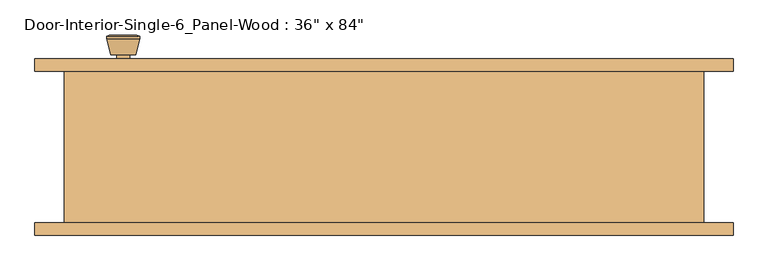
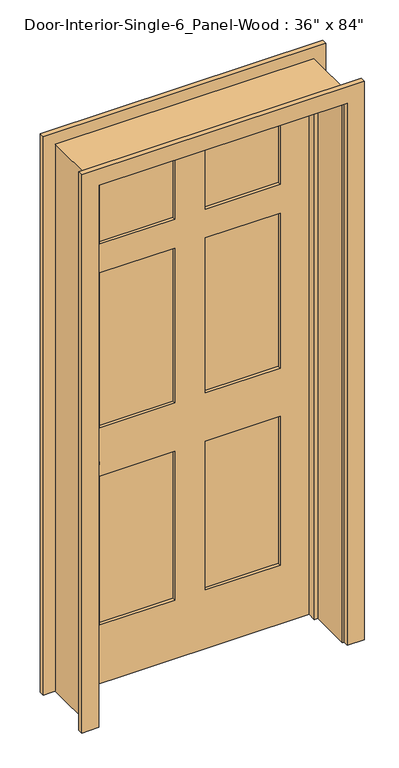
"""IFC4 building model written with IfcOpenShell, lengths in millimetres: door geometry."""

from ifc_helpers import new_model, si_unit, point, frame, frame_2d, origin, place, context, project, spatial, polyline, circle_curve, trimmed, segment, composite_curve, outline, extrude, faceted_brep, source, transform, mapped, element, save
from ifc_brep_helpers import plane_surface, cylinder_surface, revolved_surface, advanced_brep


def door_d86b6c54(model_context):
    return source(origin(), model_context, "Body", "SolidModel", [
        advanced_brep(
        [(-393.7, 70.2, 914.4), (-383.7, 70.2, 914.4), (-403.7, 70.2, 914.4), (-373.2241324, 21.2, 914.4), (-393.7, 21.2, 914.4), (-414.1758676, 21.2, 914.4), (-368.7, 23.0278681, 914.4), (-418.7, 23.0278681, 914.4), (-368.7, 26.4915463, 914.4), (-418.7, 26.4915463, 914.4), (-375.063764, 51.2, 914.4), (-412.336236, 51.2, 914.4), (-383.7, 51.2, 914.4), (-403.7, 51.2, 914.4)],
        [
            (0, 1),
            (1, 2, circle_curve(frame((-393.7, 70.2, 914.4), z_axis=(0.0, 1.0, 0.0), x_axis=(-1.0, 0.0, 0.0)), 10.0)),
            (2, 0),
            (2, 1, circle_curve(frame((-393.7, 70.2, 914.4), z_axis=(0.0, 1.0, 0.0), x_axis=(-1.0, 0.0, 0.0)), 10.0)),
            (3, 4),
            (4, 5),
            (5, 3, circle_curve(frame((-393.7, 21.2, 914.4), z_axis=(0.0, -1.0, 0.0), x_axis=(-1.0, 0.0, 0.0)), 20.4758676)),
            (3, 5, circle_curve(frame((-393.7, 21.2, 914.4), z_axis=(0.0, -1.0, 0.0), x_axis=(-1.0, 0.0, 0.0)), 20.4758676)),
            (6, 3),
            (5, 7),
            (7, 6, circle_curve(frame((-393.7, 23.0278681, 914.4), z_axis=(0.0, -1.0, 0.0), x_axis=(-1.0, 0.0, 0.0)), 25.0)),
            (6, 7, circle_curve(frame((-393.7, 23.0278681, 914.4), z_axis=(0.0, -1.0, 0.0), x_axis=(-1.0, 0.0, 0.0)), 25.0)),
            (8, 6),
            (7, 9),
            (9, 8, circle_curve(frame((-393.7, 26.4915463, 914.4), z_axis=(0.0, -1.0, 0.0), x_axis=(-1.0, 0.0, 0.0)), 25.0)),
            (8, 9, circle_curve(frame((-393.7, 26.4915463, 914.4), z_axis=(0.0, -1.0, 0.0), x_axis=(-1.0, 0.0, 0.0)), 25.0)),
            (10, 8),
            (9, 11),
            (11, 10, circle_curve(frame((-393.7, 51.2, 914.4), z_axis=(0.0, -1.0, 0.0), x_axis=(-1.0, 0.0, 0.0)), 18.636236)),
            (10, 11, circle_curve(frame((-393.7, 51.2, 914.4), z_axis=(0.0, -1.0, 0.0), x_axis=(-1.0, 0.0, 0.0)), 18.636236)),
            (12, 10),
            (11, 13),
            (13, 12, circle_curve(frame((-393.7, 51.2, 914.4), z_axis=(0.0, -1.0, 0.0), x_axis=(-1.0, 0.0, 0.0)), 10.0)),
            (12, 13, circle_curve(frame((-393.7, 51.2, 914.4), z_axis=(0.0, -1.0, 0.0), x_axis=(-1.0, 0.0, 0.0)), 10.0)),
            (1, 12),
            (13, 2),
        ],
        [
            plane_surface(frame((-393.7, 70.2, 914.4), z_axis=(0.0, 1.0, 0.0), x_axis=(-1.0, 0.0, 0.0))),
            plane_surface(frame((-393.7, 21.2, 914.4), z_axis=(0.0, -1.0, 0.0), x_axis=(-1.0, 0.0, 0.0))),
            revolved_surface(polyline([(-414.1758676, 21.2, 914.4), (-418.7, 23.0278681, 914.4)]), (-393.7, 70.2, 914.4), (0.0, 1.0, 0.0)),
            cylinder_surface(frame((-393.7, 70.2, 914.4), z_axis=(0.0, 1.0, 0.0), x_axis=(-1.0, 0.0, 0.0)), 25.0),
            revolved_surface(polyline([(-418.7, 26.4915463, 914.4), (-412.336236, 51.2, 914.4)]), (-393.7, 70.2, 914.4), (0.0, 1.0, 0.0)),
            plane_surface(frame((-393.7, 51.2, 914.4), z_axis=(0.0, 1.0, 0.0), x_axis=(-1.0, 0.0, 0.0))),
            cylinder_surface(frame((-393.7, 70.2, 914.4), z_axis=(0.0, 1.0, 0.0), x_axis=(-1.0, 0.0, 0.0)), 10.0),
        ],
        [
            (0, [[1, 2, 3]]),
            (0, [[-3, 4, -1]]),
            (1, [[5, 6, 7]]),
            (1, [[-6, -5, 8]]),
            (2, [[9, -7, 10, 11]]),
            (2, [[-10, -8, -9, 12]]),
            (3, [[13, -11, 14, 15]]),
            (3, [[-14, -12, -13, 16]]),
            (4, [[17, -15, 18, 19]]),
            (4, [[-18, -16, -17, 20]]),
            (5, [[21, -19, 22, 23]]),
            (5, [[-22, -20, -21, 24]]),
            (6, [[25, -23, 26, -2]]),
            (6, [[-26, -24, -25, -4]]),
        ],
    ),
        extrude(outline(composite_curve([segment(trimmed(circle_curve(frame_2d((914.4, -393.7)), 30.0), [point((914.4, -423.7))], [point((914.4, -363.7))], False, "CARTESIAN"), True, "CONTINUOUS"), segment(trimmed(circle_curve(frame_2d((914.4, -393.7)), 30.0), [point((914.4, -363.7))], [point((914.4, -423.7))], False, "CARTESIAN"), True, "CONTINUOUS")], self_intersect=False)), frame((0.0, 70.2, 0.0), z_axis=(0.0, 1.0, 0.0), x_axis=(0.0, 0.0, 1.0)), (0.0, 0.0, 1.0), 6.0),
        advanced_brep(
        [(-393.7, 117.125, 914.4), (-403.7, 117.125, 914.4), (-383.7, 117.125, 914.4), (-373.2241324, 166.125, 914.4), (-414.1758676, 166.125, 914.4), (-393.7, 166.125, 914.4), (-368.7, 164.2971319, 914.4), (-418.7, 164.2971319, 914.4), (-368.7, 160.8334537, 914.4), (-418.7, 160.8334537, 914.4), (-375.063764, 136.125, 914.4), (-412.336236, 136.125, 914.4), (-383.7, 136.125, 914.4), (-403.7, 136.125, 914.4)],
        [
            (0, 1),
            (1, 2, circle_curve(frame((-393.7, 117.125, 914.4), z_axis=(0.0, -1.0, 0.0), x_axis=(-1.0, 0.0, 0.0)), 10.0)),
            (2, 0),
            (2, 1, circle_curve(frame((-393.7, 117.125, 914.4), z_axis=(0.0, -1.0, 0.0), x_axis=(-1.0, 0.0, 0.0)), 10.0)),
            (3, 4, circle_curve(frame((-393.7, 166.125, 914.4), z_axis=(0.0, 1.0, 0.0), x_axis=(-1.0, 0.0, 0.0)), 20.4758676)),
            (4, 5),
            (5, 3),
            (4, 3, circle_curve(frame((-393.7, 166.125, 914.4), z_axis=(0.0, 1.0, 0.0), x_axis=(-1.0, 0.0, 0.0)), 20.4758676)),
            (6, 7, circle_curve(frame((-393.7, 164.2971319, 914.4), z_axis=(0.0, 1.0, 0.0), x_axis=(-1.0, 0.0, 0.0)), 25.0)),
            (7, 4),
            (3, 6),
            (7, 6, circle_curve(frame((-393.7, 164.2971319, 914.4), z_axis=(0.0, 1.0, 0.0), x_axis=(-1.0, 0.0, 0.0)), 25.0)),
            (8, 9, circle_curve(frame((-393.7, 160.8334537, 914.4), z_axis=(0.0, 1.0, 0.0), x_axis=(-1.0, 0.0, 0.0)), 25.0)),
            (9, 7),
            (6, 8),
            (9, 8, circle_curve(frame((-393.7, 160.8334537, 914.4), z_axis=(0.0, 1.0, 0.0), x_axis=(-1.0, 0.0, 0.0)), 25.0)),
            (10, 11, circle_curve(frame((-393.7, 136.125, 914.4), z_axis=(0.0, 1.0, 0.0), x_axis=(-1.0, 0.0, 0.0)), 18.636236)),
            (11, 9),
            (8, 10),
            (11, 10, circle_curve(frame((-393.7, 136.125, 914.4), z_axis=(0.0, 1.0, 0.0), x_axis=(-1.0, 0.0, 0.0)), 18.636236)),
            (12, 13, circle_curve(frame((-393.7, 136.125, 914.4), z_axis=(0.0, 1.0, 0.0), x_axis=(-1.0, 0.0, 0.0)), 10.0)),
            (13, 11),
            (10, 12),
            (13, 12, circle_curve(frame((-393.7, 136.125, 914.4), z_axis=(0.0, 1.0, 0.0), x_axis=(-1.0, 0.0, 0.0)), 10.0)),
            (1, 13),
            (12, 2),
        ],
        [
            plane_surface(frame((-393.7, 117.125, 914.4), z_axis=(0.0, -1.0, 0.0), x_axis=(-1.0, 0.0, 0.0))),
            plane_surface(frame((-393.7, 166.125, 914.4), z_axis=(0.0, 1.0, 0.0), x_axis=(-1.0, 0.0, 0.0))),
            revolved_surface(polyline([(-414.1758676, 166.125, 914.4), (-418.7, 164.2971319, 914.4)]), (-393.7, 117.125, 914.4), (0.0, -1.0, 0.0)),
            cylinder_surface(frame((-393.7, 117.125, 914.4), z_axis=(0.0, -1.0, 0.0), x_axis=(-1.0, 0.0, 0.0)), 25.0),
            revolved_surface(polyline([(-418.7, 160.8334537, 914.4), (-412.336236, 136.125, 914.4)]), (-393.7, 117.125, 914.4), (0.0, -1.0, 0.0)),
            plane_surface(frame((-393.7, 136.125, 914.4), z_axis=(0.0, -1.0, 0.0), x_axis=(-1.0, 0.0, 0.0))),
            cylinder_surface(frame((-393.7, 117.125, 914.4), z_axis=(0.0, -1.0, 0.0), x_axis=(-1.0, 0.0, 0.0)), 10.0),
        ],
        [
            (0, [[1, 2, 3]]),
            (0, [[-3, 4, -1]]),
            (1, [[5, 6, 7]]),
            (1, [[8, -7, -6]]),
            (2, [[9, 10, -5, 11]]),
            (2, [[12, -11, -8, -10]]),
            (3, [[13, 14, -9, 15]]),
            (3, [[16, -15, -12, -14]]),
            (4, [[17, 18, -13, 19]]),
            (4, [[20, -19, -16, -18]]),
            (5, [[21, 22, -17, 23]]),
            (5, [[24, -23, -20, -22]]),
            (6, [[-2, 25, -21, 26]]),
            (6, [[-4, -26, -24, -25]]),
        ],
    ),
        extrude(outline(composite_curve([segment(trimmed(circle_curve(frame_2d((914.4, -393.7)), 30.0), [point((914.4, -423.7))], [point((914.4, -363.7))], False, "CARTESIAN"), True, "CONTINUOUS"), segment(trimmed(circle_curve(frame_2d((914.4, -393.7)), 30.0), [point((914.4, -363.7))], [point((914.4, -423.7))], False, "CARTESIAN"), True, "CONTINUOUS")], self_intersect=False)), frame((0.0, 111.125, 0.0), z_axis=(0.0, 1.0, 0.0), x_axis=(0.0, 0.0, 1.0)), (0.0, 0.0, 1.0), 6.0),
        faceted_brep([(482.6, 111.125, 0.0), (482.6, -117.475, 0.0), (457.2, -117.475, 0.0), (457.2, 41.275, 0.0), (444.5, 41.275, 0.0), (444.5, 76.2, 0.0), (457.2, 76.2, 0.0), (457.2, 111.125, 0.0), (482.6, 111.125, 2159.0), (482.6, -117.475, 2159.0), (-482.6, -117.475, 2159.0), (-482.6, -117.475, 0.0), (-457.2, -117.475, 0.0), (-457.2, -117.475, 2133.6), (457.2, -117.475, 2133.6), (457.2, 41.275, 2133.6), (-457.2, 41.275, 2133.6), (-457.2, 41.275, 0.0), (-444.5, 41.275, 0.0), (-444.5, 41.275, 2120.9), (444.5, 41.275, 2120.9), (444.5, 76.2, 2120.9), (-444.5, 76.2, 2120.9), (-444.5, 76.2, 0.0), (-457.2, 76.2, 0.0), (-457.2, 76.2, 2133.6), (457.2, 76.2, 2133.6), (457.2, 111.125, 2133.6), (-457.2, 111.125, 2133.6), (-457.2, 111.125, 0.0), (-482.6, 111.125, 0.0), (-482.6, 111.125, 2159.0)], [[[0, 1, 2, 3, 4, 5, 6, 7]], [[1, 0, 8, 9]], [[2, 1, 9, 10, 11, 12, 13, 14]], [[3, 2, 14, 15]], [[4, 3, 15, 16, 17, 18, 19, 20]], [[5, 4, 20, 21]], [[6, 5, 21, 22, 23, 24, 25, 26]], [[7, 6, 26, 27]], [[0, 7, 27, 28, 29, 30, 31, 8]], [[9, 8, 31, 10]], [[15, 14, 13, 16]], [[21, 20, 19, 22]], [[27, 26, 25, 28]], [[30, 29, 24, 23, 18, 17, 12, 11]], [[10, 31, 30, 11]], [[16, 13, 12, 17]], [[22, 19, 18, 23]], [[28, 25, 24, 29]]]),
        extrude(outline(polyline([(2133.6, -457.2), (0.0, -457.2), (0.0, 457.2), (2133.6, 457.2), (2133.6, -457.2)]), holes=[polyline([(2014.5375, 57.15), (2014.5375, 336.55), (1735.1375, 336.55), (1735.1375, 57.15), (2014.5375, 57.15)]), polyline([(1620.8375, 336.55), (1009.65, 336.55), (1009.65, 57.15), (1620.8375, 57.15), (1620.8375, 336.55)]), polyline([(1009.65, -57.15), (1009.65, -336.55), (1620.8375, -336.55), (1620.8375, -57.15), (1009.65, -57.15)]), polyline([(1735.1375, -336.55), (2014.5375, -336.55), (2014.5375, -57.15), (1735.1375, -57.15), (1735.1375, -336.55)]), polyline([(819.15, 57.15), (819.15, 336.55), (231.775, 336.55), (231.775, 57.15), (819.15, 57.15)]), polyline([(231.775, -57.15), (231.775, -336.55), (819.15, -336.55), (819.15, -57.15), (231.775, -57.15)])]), frame((0.0, 76.2, 0.0), z_axis=(0.0, 1.0, 0.0), x_axis=(0.0, 0.0, 1.0)), (0.0, 0.0, 1.0), 34.925),
        extrude(outline(polyline([(336.55, 87.8416667), (57.15, 87.8416667), (57.15, 99.4833333), (336.55, 99.4833333), (336.55, 87.8416667)])), frame((0.0, 0.0, 1735.1375), z_axis=(0.0, 0.0, 1.0), x_axis=(1.0, 0.0, 0.0)), (0.0, 0.0, 1.0), 279.4),
        extrude(outline(polyline([(336.55, 87.8416667), (57.15, 87.8416667), (57.15, 99.4833333), (336.55, 99.4833333), (336.55, 87.8416667)])), frame((0.0, 0.0, 1009.65), z_axis=(0.0, 0.0, 1.0), x_axis=(1.0, 0.0, 0.0)), (0.0, 0.0, 1.0), 611.1875),
        extrude(outline(polyline([(-57.15, 87.8416667), (-336.55, 87.8416667), (-336.55, 99.4833333), (-57.15, 99.4833333), (-57.15, 87.8416667)])), frame((0.0, 0.0, 1009.65), z_axis=(0.0, 0.0, 1.0), x_axis=(1.0, 0.0, 0.0)), (0.0, 0.0, 1.0), 611.1875),
        extrude(outline(polyline([(-57.15, 87.8416667), (-336.55, 87.8416667), (-336.55, 99.4833333), (-57.15, 99.4833333), (-57.15, 87.8416667)])), frame((0.0, 0.0, 1735.1375), z_axis=(0.0, 0.0, 1.0), x_axis=(1.0, 0.0, 0.0)), (0.0, 0.0, 1.0), 279.4),
        extrude(outline(polyline([(336.55, 87.8416667), (57.15, 87.8416667), (57.15, 99.4833333), (336.55, 99.4833333), (336.55, 87.8416667)])), frame((0.0, 0.0, 231.775), z_axis=(0.0, 0.0, 1.0), x_axis=(1.0, 0.0, 0.0)), (0.0, 0.0, 1.0), 587.375),
        extrude(outline(polyline([(-57.15, 87.8416667), (-336.55, 87.8416667), (-336.55, 99.4833333), (-57.15, 99.4833333), (-57.15, 87.8416667)])), frame((0.0, 0.0, 231.775), z_axis=(0.0, 0.0, 1.0), x_axis=(1.0, 0.0, 0.0)), (0.0, 0.0, 1.0), 587.375),
        extrude(outline(polyline([(0.0, 463.55), (0.0, 527.05), (2203.45, 527.05), (2203.45, -527.05), (0.0, -527.05), (0.0, -463.55), (2139.95, -463.55), (2139.95, 463.55), (0.0, 463.55)])), frame((0.0, 111.125, 0.0), z_axis=(0.0, 1.0, 0.0), x_axis=(0.0, 0.0, 1.0)), (0.0, 0.0, 1.0), 19.05),
        extrude(outline(polyline([(0.0, 463.55), (0.0, 527.05), (2203.45, 527.05), (2203.45, -527.05), (0.0, -527.05), (0.0, -463.55), (2139.95, -463.55), (2139.95, 463.55), (0.0, 463.55)])), frame((0.0, -136.525, 0.0), z_axis=(0.0, 1.0, 0.0), x_axis=(0.0, 0.0, 1.0)), (0.0, 0.0, 1.0), 19.05),
    ])


if __name__ == "__main__":
    model = new_model("IFC4")
    model_context = context("Model", 3, world=origin())
    ifc_project = project(units=[si_unit("LENGTHUNIT", "METRE", prefix="MILLI")], contexts=[model_context])
    site = spatial("IfcSite", under=ifc_project)
    building = spatial("IfcBuilding", under=site)
    placement = place(None, origin())
    door_shape = door_d86b6c54(model_context)
    element("IfcDoor", 1, ObjectType="Door-Interior-Single-6_Panel-Wood : 36\" x 84\"", at=placement, inside=building, context=model_context, shape_type="MappedRepresentation", body=[
        mapped(door_shape, transform((0.0, 0.0, 0.0), x_axis=(1.0, 0.0, 0.0), y_axis=(0.0, 1.0, 0.0), z_axis=(0.0, 0.0, 1.0))),
    ])
    save(model, "model.ifc")

# Revit data of these elements
# Type "Door-Interior-Single-6_Panel-Wood : 36\" x 84\""
#   Type Mark = "9"
#   Assembly Code = "C1020300"
#   Analytic Construction = "Wooden"
#   Top Rail = 0' - 4 11/16"
#   Top Panel = 0' - 11"
#   Thickness = 0' - 1 3/8"
#   Thermal Resistance (R) = 2.5876 (h·ft²·°F)/BTU
#   Swing Angle [instance default] = 90.00°
#   Stiles = 0' - 4 3/4"
#   Rough Width = 3' - 2"
#   Rough Height = 7' - 1"
#   Mullion = 0' - 4 1/2"
#   Lock Rail = 0' - 7 1/2"
#   Intermediate Rail = 0' - 4 1/2"
#   Height = 7' - 0"
#   Width = 3' - 0"
#   Heat Transfer Coefficient (U) = 0.3865 BTU/(h·ft²·°F)
#   Bottom Rail = 0' - 9 1/8"
#   Trim Material = Cherry
#   Panel Material = Cherry
#   Frame Material = Cherry
#   Door Handle Material = Aluminum
#   Visual Light Transmittance = 0
#   Solar Heat Gain Coefficient = 0
#   Wall Closure = (empty or 0)
#   Function = (empty or 0)
# Element 1 (IfcDoor, "Door-Interior-Single-6_Panel-Wood : 36\" x 84\"")
#   Materials on its faces: "Cherry", "Aluminum"
# Materials
#   "Cherry": class "Wood", colour RGB 226 177 128, transparency 0, Description = "Prunus Serotina", Cost = 0
#   "Aluminum": class "Metal", colour RGB 247 247 247, transparency 0, Description = "Aluminum 6061", Cost = 0
